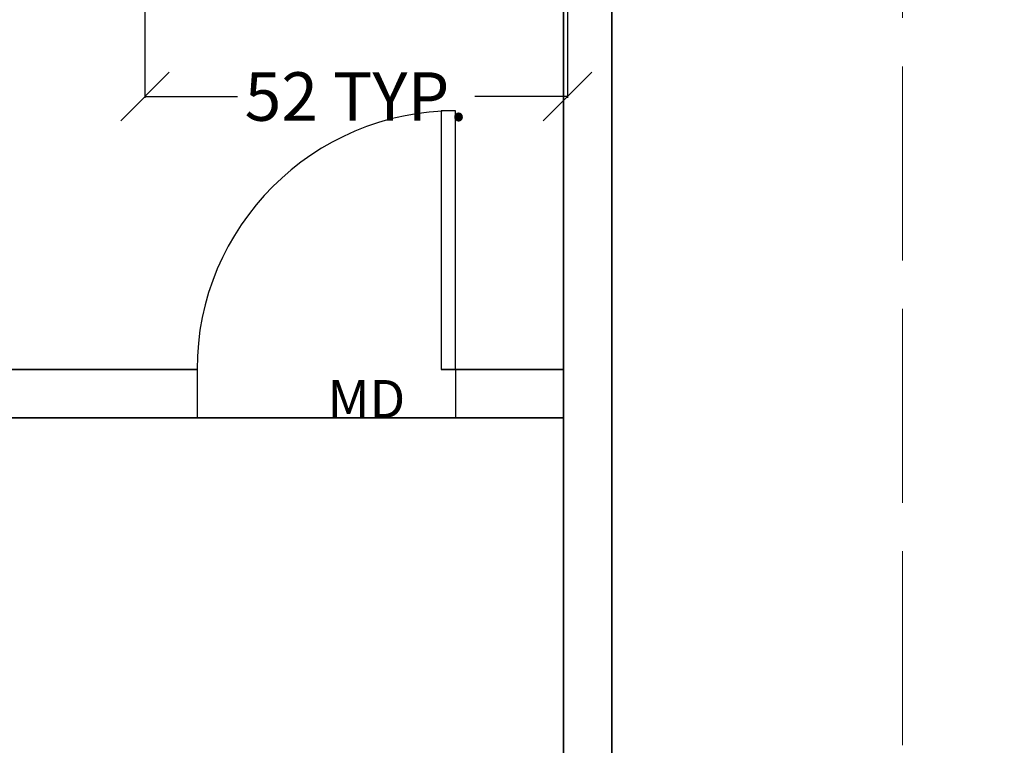
# Model space of a CAD drawing. Units: inches. Extents: x -1198 to -69, y -512 to 437.
# Tile 43 of 50: x -444 to -322, y -85 to 5. Entities that reach past the tile are written whole.
import ezdxf

# ---------------------------------------------------------------- set-up
doc = ezdxf.new("R2010")
doc.units = ezdxf.units.IN
doc.header["$MEASUREMENT"] = 0
doc.linetypes.add('ACAD_ISO02W100', pattern=[15, 12, -3])
for name, color, linetype, lineweight in [('A-ANNO-DIMS', 2, 'Continuous', 18), ('A-ANNO-SYMB', 7, 'Continuous', 18), ('A-WALL', 7, 'Continuous', 35), ('C-PROP', 141, 'ACAD_ISO02W100', 18), ('Doors', 140, 'Continuous', 25)]:
    doc.layers.add(name, color=color, linetype=linetype, lineweight=lineweight)
doc.styles.get("Standard").update_dxf_attribs({"font": 'arial.ttf'})
doc.dimstyles.get("Standard").update_dxf_attribs({"dimtxt": 6, "dimasz": 6, "dimexe": 0.18, "dimexo": 0.0625, "dimgap": 0.09, "dimtad": 0, "dimtih": 1, "dimtoh": 1, "dimdec": 0, "dimzin": 0, "dimdsep": 46, "dimlunit": 4, "dimtxsty": 'Standard', "dimblk": 'OBLIQUE', "dimcen": 0.09, "dimadec": 0, "dimazin": 0, "dimtfac": 1, "dimtdec": 0, "dimtofl": 0, "dimtmove": 0, "dimatfit": 3, "dimfxl": 1, "dimtolj": 1, "dimtzin": 0, "dimarcsym": 0})

# ---------------------------------------------------------------- blocks, each defined once
blk = doc.blocks.new('*U5')
for p, q in [((0, 0), (0, -6)), ((-32, 0), (-32, -6))]:
    blk.add_line(p, q)
blk.add_lwpolyline([(0, 0), (0, 32), (-1.75, 32), (-1.75, 0)], close=True)
blk.add_arc((0, 0), 32, 90, 180)
blk = doc.blocks.new('_Oblique')
at = {"color": 0, "linetype": 'ByBlock', "lineweight": -2}
blk.add_line((-0.5, -0.5), (0.5, 0.5), dxfattribs=at)
blk = doc.blocks.new('*D53')
at = {"layer": 'A-ANNO-DIMS', "color": 0, "lineweight": -2, "ltscale": 10, "transparency": 16777216}
for p, q in [((-428.58, 9.92), (-428.58, -4.68)), ((-376.25, 9.92), (-376.25, -4.68)), ((-428.58, -4.5), (-417.11, -4.5)), ((-376.25, -4.5), (-387.72, -4.5))]:
    blk.add_line(p, q, dxfattribs=at)
at = {"layer": 'DEFPOINTS', "color": 0, "ltscale": 10, "transparency": 16777216}
for p in [(-428.58, 9.98), (-376.25, 9.98), (-376.25, -4.5)]:
    blk.add_point(p, dxfattribs=at)
at = {"layer": 'A-ANNO-DIMS', "color": 0, "lineweight": -2, "ltscale": 10, "transparency": 16777216, "xscale": 6, "yscale": 6, "zscale": 6, "rotation": 180}
blk.add_blockref('_Oblique', (-428.58, -4.5), dxfattribs=at)
at = {"layer": 'A-ANNO-DIMS', "color": 0, "lineweight": -2, "ltscale": 10, "transparency": 16777216, "xscale": 6, "yscale": 6, "zscale": 6}
blk.add_blockref('_Oblique', (-376.25, -4.5), dxfattribs=at)
at = {"layer": 'A-ANNO-DIMS', "color": 0, "ltscale": 10, "transparency": 16777216, "insert": (-402.42, -4.5), "char_height": 6, "attachment_point": 5}
blk.add_mtext('\\A1;52 TYP.', dxfattribs=at)
blk = doc.blocks.new('*D63')
at = {"layer": 'A-ANNO-DIMS', "color": 0, "lineweight": -2, "ltscale": 10, "transparency": 16777216}
for p, q in [((-370.69, 263.23), (-79.37, 263.23)), ((-79.55, 263.23), (-79.55, 20.38)), ((-79.55, -228.77), (-79.55, 14.07)), ((-370.69, -228.77), (-79.37, -228.77))]:
    blk.add_line(p, q, dxfattribs=at)
at = {"layer": 'DEFPOINTS', "color": 0, "ltscale": 10, "transparency": 16777216}
for p in [(-370.75, 263.23), (-79.55, 263.23), (-370.75, -228.77)]:
    blk.add_point(p, dxfattribs=at)
at = {"layer": 'A-ANNO-DIMS', "color": 0, "lineweight": -2, "ltscale": 10, "transparency": 16777216, "xscale": 6, "yscale": 6, "zscale": 6}
for p, rotation in [((-79.55, 263.23), 90), ((-79.55, -228.77), 270)]:
    blk.add_blockref('_Oblique', p, dxfattribs=dict(at, rotation=rotation))
at = {"layer": 'A-ANNO-DIMS', "color": 0, "ltscale": 10, "transparency": 16777216, "insert": (-79.55, 17.23), "char_height": 6, "attachment_point": 5}
blk.add_mtext('\\A1;492', dxfattribs=at)
blk = doc.blocks.new('*D75')
at = {"layer": 'A-ANNO-DIMS', "color": 0, "lineweight": -2, "ltscale": 10, "transparency": 16777216}
for p, q in [((-376.81, -44.27), (-1188.2, -44.27)), ((-1188.02, -44.27), (-1188.02, -133.37)), ((-1188.02, -228.77), (-1188.02, -139.68)), ((-370.81, -228.77), (-1188.2, -228.77))]:
    blk.add_line(p, q, dxfattribs=at)
at = {"layer": 'DEFPOINTS', "color": 0, "ltscale": 10, "transparency": 16777216}
for p in [(-1188.02, -44.27), (-376.75, -44.27), (-370.75, -228.77)]:
    blk.add_point(p, dxfattribs=at)
at = {"layer": 'A-ANNO-DIMS', "color": 0, "lineweight": -2, "ltscale": 10, "transparency": 16777216, "xscale": 6, "yscale": 6, "zscale": 6}
for p, rotation in [((-1188.02, -44.27), 90), ((-1188.02, -228.77), 270)]:
    blk.add_blockref('_Oblique', p, dxfattribs=dict(at, rotation=rotation))
at = {"layer": 'A-ANNO-DIMS', "color": 0, "ltscale": 10, "transparency": 16777216, "insert": (-1188.02, -136.52), "char_height": 6, "attachment_point": 5}
blk.add_mtext('\\A1;184.5', dxfattribs=at)

msp = doc.modelspace()

# ---------------------------------------------------------------- linework, layer by layer
at = {"layer": 'A-WALL', "ltscale": 10}
for p, q in [((-370.7509, -228.7723), (-370.7509, 263.2277)), ((-376.7509, -222.7723), (-376.7509, 257.2277)), ((-422.1319, -38.2723), (-565.7509, -38.2723)), ((-376.7509, -38.2723), (-391.8819, -38.2723)), ((-376.7509, -44.2723), (-565.7509, -44.2723))]:
    msp.add_line(p, q, dxfattribs=at)
at = {"layer": 'C-PROP', "ltscale": 2}
msp.add_lwpolyline([(-1054.7509, 299.2277), (-334.7509, 299.2277), (-334.7509, -264.7723), (-1054.7509, -264.7723)], close=True, dxfattribs=at)

# ---------------------------------------------------------------- block references
at = {"layer": 'Doors'}
msp.add_blockref('*U5', (-390.1319, -38.2723), dxfattribs=at)

# ---------------------------------------------------------------- texts
at = {"layer": 'A-ANNO-SYMB', "ltscale": 10}
msp.add_text('MD', height=4.69957, dxfattribs=at).set_placement((-405.9671, -44.2723))

# ---------------------------------------------------------------- dimensions: what is measured, and where the dimension line sits
at = {"layer": 'A-ANNO-DIMS', "ltscale": 10}
for base, p2, override, picture, middle in [((-79.5507, 263.2277), (-370.7509, 263.2277), {"dimdec": 0, "dimlfac": 1, "dimrnd": 0, "dimzin": 0, "dimdsep": 46, "dimlunit": 2}, '*D63', (-79.5507, 17.2277)), ((-1188.0248, -44.2723), (-376.7509, -44.2723), {"dimdec": 1, "dimlfac": 1, "dimrnd": 0, "dimzin": 0, "dimdsep": 46, "dimlunit": 2}, '*D75', (-1188.0248, -136.5223))]:
    dim = msp.add_linear_dim(base=base, p1=(-370.7509, -228.7723), p2=p2, angle=90, dimstyle='Standard', override=override, dxfattribs=at)
    dim.commit()
    dim.dimension.update_dxf_attribs({"geometry": picture, "text_midpoint": middle})
dim = msp.add_linear_dim(base=(-376.2476, -4.5045), p1=(-428.5837, 9.981), p2=(-376.2476, 9.981), angle=0, text='<> TYP.', dimstyle='Standard', override={"dimdec": 0, "dimlfac": 1, "dimrnd": 0, "dimzin": 0, "dimdsep": 46, "dimlunit": 2}, dxfattribs=at)
dim.commit()
dim.dimension.update_dxf_attribs({"geometry": '*D53', "text_midpoint": (-402.4157, -4.5045)})

doc.saveas('drawing.dxf')
